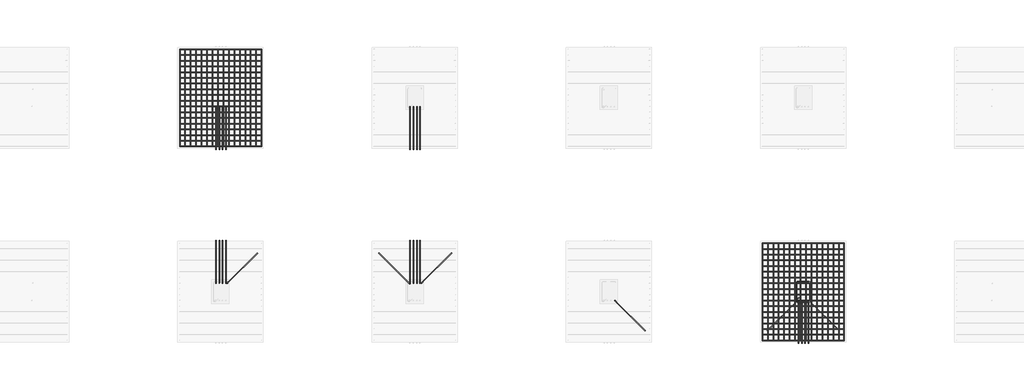
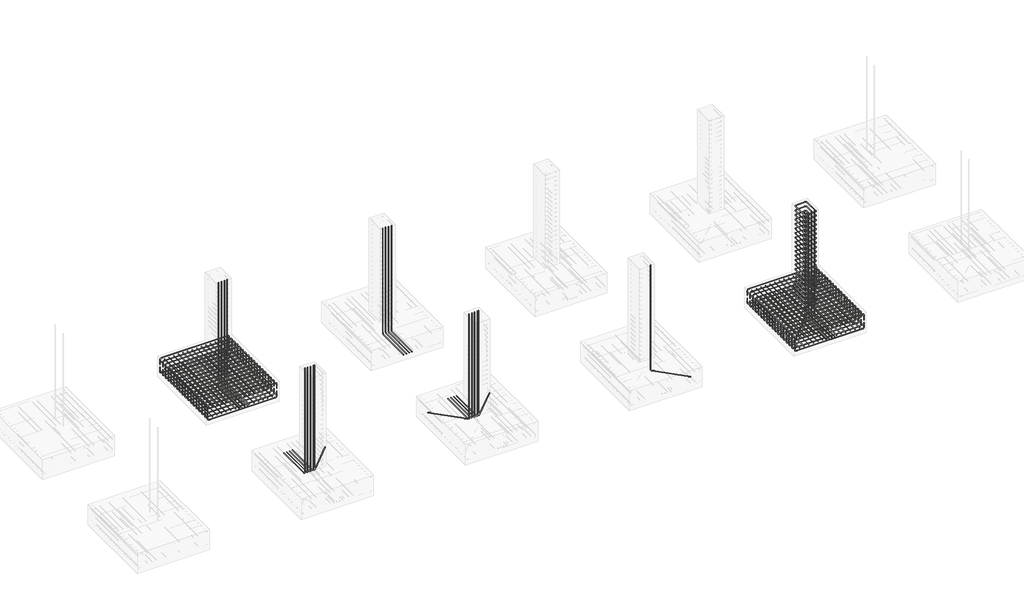
# One storey, part 8 of 33: 20 reinforcing bars.
"""IFC4 building model written with IfcOpenShell, lengths in millimetres."""

from ifc_helpers import new_model, si_unit, point, frame, origin, place, context, project, spatial, polyline, circle_curve, trimmed, segment, composite_curve, source, transform, mapped, element, save
from ifc_brep_helpers import swept_disk

model = new_model("IFC4")

# Units and contexts
model_context = context("Model", 3, world=origin())
ifc_project = project(units=[si_unit("LENGTHUNIT", "METRE", prefix="MILLI")], contexts=[model_context])

# Site, building, storey
site = spatial("IfcSite", under=ifc_project)
building = spatial("IfcBuilding", under=site)
storey = spatial("IfcBuildingStorey", under=building, Elevation=-3000.0)

# Reinforcing bars
placement = place(None, origin())
reinforcing_bar_shape = source(origin(), model_context, "Body", "SolidModel", [
    swept_disk(composite_curve([segment(polyline([(14306.5357258, -7044.0608134, -3240.0), (14306.5357258, -7044.0608134, -3092.7)]), True, "CONTINUOUS"), segment(trimmed(circle_curve(frame((14352.8857258, -7044.0608134, -3092.7), z_axis=(0.0, 1.0, 0.0), x_axis=(-46.350000000000364, 0.0, 0.0)), 46.35), [point((14306.5357258, -7044.0608134, -3092.7))], [point((14352.8857258, -7044.0608134, -3046.35))], True, "CARTESIAN"), True, "CONTINUOUS"), segment(polyline([(14352.8857258, -7044.0608134, -3046.35), (16367.4857258, -7044.0608134, -3046.35)]), True, "CONTINUOUS"), segment(trimmed(circle_curve(frame((16367.4857258, -7044.0608134, -3092.7), z_axis=(0.0, 1.0, 0.0), x_axis=(0.0, 0.0, 46.34999999999991)), 46.35), [point((16367.4857258, -7044.0608134, -3046.35))], [point((16413.8357258, -7044.0608134, -3092.7))], True, "CARTESIAN"), True, "CONTINUOUS"), segment(polyline([(16413.8357258, -7044.0608134, -3092.7), (16413.8357258, -7044.0608134, -3240.0)]), True, "CONTINUOUS")], self_intersect=False), 6.35),
])
element("IfcReinforcingBar", 1, at=placement, inside=storey, context=model_context, shape_type="MappedRepresentation", body=[
    mapped(reinforcing_bar_shape, transform((0.0, 0.0, 0.0), x_axis=(1.0, 0.0, 0.0), y_axis=(0.0, 1.0, 0.0), z_axis=(0.0, 0.0, 1.0))),
    mapped(reinforcing_bar_shape, transform((0.0, -147.4882353, 0.0), x_axis=(1.0, 0.0, 0.0), y_axis=(0.0, 1.0, 0.0), z_axis=(0.0, 0.0, 1.0))),
    mapped(reinforcing_bar_shape, transform((0.0, -294.9764706, 0.0), x_axis=(1.0, 0.0, 0.0), y_axis=(0.0, 1.0, 0.0), z_axis=(0.0, 0.0, 1.0))),
    mapped(reinforcing_bar_shape, transform((0.0, -442.4647059, 0.0), x_axis=(1.0, 0.0, 0.0), y_axis=(0.0, 1.0, 0.0), z_axis=(0.0, 0.0, 1.0))),
    mapped(reinforcing_bar_shape, transform((0.0, -589.9529412, 0.0), x_axis=(1.0, 0.0, 0.0), y_axis=(0.0, 1.0, 0.0), z_axis=(0.0, 0.0, 1.0))),
    mapped(reinforcing_bar_shape, transform((0.0, -737.4411765, 0.0), x_axis=(1.0, 0.0, 0.0), y_axis=(0.0, 1.0, 0.0), z_axis=(0.0, 0.0, 1.0))),
    mapped(reinforcing_bar_shape, transform((0.0, -884.9294118, 0.0), x_axis=(1.0, 0.0, 0.0), y_axis=(0.0, 1.0, 0.0), z_axis=(0.0, 0.0, 1.0))),
    mapped(reinforcing_bar_shape, transform((0.0, -1032.4176471, 0.0), x_axis=(1.0, 0.0, 0.0), y_axis=(0.0, 1.0, 0.0), z_axis=(0.0, 0.0, 1.0))),
    mapped(reinforcing_bar_shape, transform((0.0, -1179.9058824, 0.0), x_axis=(1.0, 0.0, 0.0), y_axis=(0.0, 1.0, 0.0), z_axis=(0.0, 0.0, 1.0))),
    mapped(reinforcing_bar_shape, transform((0.0, -1327.3941176, 0.0), x_axis=(1.0, 0.0, 0.0), y_axis=(0.0, 1.0, 0.0), z_axis=(0.0, 0.0, 1.0))),
    mapped(reinforcing_bar_shape, transform((0.0, -1474.8823529, 0.0), x_axis=(1.0, 0.0, 0.0), y_axis=(0.0, 1.0, 0.0), z_axis=(0.0, 0.0, 1.0))),
    mapped(reinforcing_bar_shape, transform((0.0, -1622.3705882, 0.0), x_axis=(1.0, 0.0, 0.0), y_axis=(0.0, 1.0, 0.0), z_axis=(0.0, 0.0, 1.0))),
    mapped(reinforcing_bar_shape, transform((0.0, -1769.8588235, 0.0), x_axis=(1.0, 0.0, 0.0), y_axis=(0.0, 1.0, 0.0), z_axis=(0.0, 0.0, 1.0))),
    mapped(reinforcing_bar_shape, transform((0.0, -1917.3470588, 0.0), x_axis=(1.0, 0.0, 0.0), y_axis=(0.0, 1.0, 0.0), z_axis=(0.0, 0.0, 1.0))),
    mapped(reinforcing_bar_shape, transform((0.0, -2064.8352941, 0.0), x_axis=(1.0, 0.0, 0.0), y_axis=(0.0, 1.0, 0.0), z_axis=(0.0, 0.0, 1.0))),
    mapped(reinforcing_bar_shape, transform((0.0, -2212.3235294, 0.0), x_axis=(1.0, 0.0, 0.0), y_axis=(0.0, 1.0, 0.0), z_axis=(0.0, 0.0, 1.0))),
    mapped(reinforcing_bar_shape, transform((0.0, -2359.8117647, 0.0), x_axis=(1.0, 0.0, 0.0), y_axis=(0.0, 1.0, 0.0), z_axis=(0.0, 0.0, 1.0))),
    mapped(reinforcing_bar_shape, transform((0.0, -2507.3, 0.0), x_axis=(1.0, 0.0, 0.0), y_axis=(0.0, 1.0, 0.0), z_axis=(0.0, 0.0, 1.0))),
])
reinforcing_bar_2_shape = source(origin(), model_context, "Body", "SolidModel", [
    swept_disk(composite_curve([segment(polyline([(16413.8357258, -7044.0608134, -3330.080452), (16413.8357258, -7044.0608134, -3477.380452)]), True, "CONTINUOUS"), segment(trimmed(circle_curve(frame((16367.4857258, -7044.0608134, -3477.380452), z_axis=(0.0, 1.0, 0.0), x_axis=(46.350000000000364, 0.0, 0.0)), 46.35), [point((16413.8357258, -7044.0608134, -3477.380452))], [point((16367.4857258, -7044.0608134, -3523.730452))], True, "CARTESIAN"), True, "CONTINUOUS"), segment(polyline([(16367.4857258, -7044.0608134, -3523.730452), (14352.8857258, -7044.0608134, -3523.730452)]), True, "CONTINUOUS"), segment(trimmed(circle_curve(frame((14352.8857258, -7044.0608134, -3477.380452), z_axis=(0.0, 1.0, 0.0), x_axis=(0.0, 0.0, -46.34999999999991)), 46.35), [point((14352.8857258, -7044.0608134, -3523.730452))], [point((14306.5357258, -7044.0608134, -3477.380452))], True, "CARTESIAN"), True, "CONTINUOUS"), segment(polyline([(14306.5357258, -7044.0608134, -3477.380452), (14306.5357258, -7044.0608134, -3330.080452)]), True, "CONTINUOUS")], self_intersect=False), 6.35),
])
element("IfcReinforcingBar", 2, at=placement, inside=storey, context=model_context, shape_type="MappedRepresentation", body=[
    mapped(reinforcing_bar_2_shape, transform((0.0, 0.0, 0.0), x_axis=(1.0, 0.0, 0.0), y_axis=(0.0, 1.0, 0.0), z_axis=(0.0, 0.0, 1.0))),
    mapped(reinforcing_bar_2_shape, transform((0.0, -147.4882353, 0.0), x_axis=(1.0, 0.0, 0.0), y_axis=(0.0, 1.0, 0.0), z_axis=(0.0, 0.0, 1.0))),
    mapped(reinforcing_bar_2_shape, transform((0.0, -294.9764706, 0.0), x_axis=(1.0, 0.0, 0.0), y_axis=(0.0, 1.0, 0.0), z_axis=(0.0, 0.0, 1.0))),
    mapped(reinforcing_bar_2_shape, transform((0.0, -442.4647059, 0.0), x_axis=(1.0, 0.0, 0.0), y_axis=(0.0, 1.0, 0.0), z_axis=(0.0, 0.0, 1.0))),
    mapped(reinforcing_bar_2_shape, transform((0.0, -589.9529412, 0.0), x_axis=(1.0, 0.0, 0.0), y_axis=(0.0, 1.0, 0.0), z_axis=(0.0, 0.0, 1.0))),
    mapped(reinforcing_bar_2_shape, transform((0.0, -737.4411765, 0.0), x_axis=(1.0, 0.0, 0.0), y_axis=(0.0, 1.0, 0.0), z_axis=(0.0, 0.0, 1.0))),
    mapped(reinforcing_bar_2_shape, transform((0.0, -884.9294118, 0.0), x_axis=(1.0, 0.0, 0.0), y_axis=(0.0, 1.0, 0.0), z_axis=(0.0, 0.0, 1.0))),
    mapped(reinforcing_bar_2_shape, transform((0.0, -1032.4176471, 0.0), x_axis=(1.0, 0.0, 0.0), y_axis=(0.0, 1.0, 0.0), z_axis=(0.0, 0.0, 1.0))),
    mapped(reinforcing_bar_2_shape, transform((0.0, -1179.9058824, 0.0), x_axis=(1.0, 0.0, 0.0), y_axis=(0.0, 1.0, 0.0), z_axis=(0.0, 0.0, 1.0))),
    mapped(reinforcing_bar_2_shape, transform((0.0, -1327.3941176, 0.0), x_axis=(1.0, 0.0, 0.0), y_axis=(0.0, 1.0, 0.0), z_axis=(0.0, 0.0, 1.0))),
    mapped(reinforcing_bar_2_shape, transform((0.0, -1474.8823529, 0.0), x_axis=(1.0, 0.0, 0.0), y_axis=(0.0, 1.0, 0.0), z_axis=(0.0, 0.0, 1.0))),
    mapped(reinforcing_bar_2_shape, transform((0.0, -1622.3705882, 0.0), x_axis=(1.0, 0.0, 0.0), y_axis=(0.0, 1.0, 0.0), z_axis=(0.0, 0.0, 1.0))),
    mapped(reinforcing_bar_2_shape, transform((0.0, -1769.8588235, 0.0), x_axis=(1.0, 0.0, 0.0), y_axis=(0.0, 1.0, 0.0), z_axis=(0.0, 0.0, 1.0))),
    mapped(reinforcing_bar_2_shape, transform((0.0, -1917.3470588, 0.0), x_axis=(1.0, 0.0, 0.0), y_axis=(0.0, 1.0, 0.0), z_axis=(0.0, 0.0, 1.0))),
    mapped(reinforcing_bar_2_shape, transform((0.0, -2064.8352941, 0.0), x_axis=(1.0, 0.0, 0.0), y_axis=(0.0, 1.0, 0.0), z_axis=(0.0, 0.0, 1.0))),
    mapped(reinforcing_bar_2_shape, transform((0.0, -2212.3235294, 0.0), x_axis=(1.0, 0.0, 0.0), y_axis=(0.0, 1.0, 0.0), z_axis=(0.0, 0.0, 1.0))),
    mapped(reinforcing_bar_2_shape, transform((0.0, -2359.8117647, 0.0), x_axis=(1.0, 0.0, 0.0), y_axis=(0.0, 1.0, 0.0), z_axis=(0.0, 0.0, 1.0))),
    mapped(reinforcing_bar_2_shape, transform((0.0, -2507.3, 0.0), x_axis=(1.0, 0.0, 0.0), y_axis=(0.0, 1.0, 0.0), z_axis=(0.0, 0.0, 1.0))),
])
reinforcing_bar_3_shape = source(origin(), model_context, "Body", "SolidModel", [
    swept_disk(composite_curve([segment(polyline([(16413.8357258, -9557.7108134, -3447.8614173), (16413.8357258, -7037.7108134, -3447.8614173)]), True, "CONTINUOUS")], self_intersect=False), 6.35),
])
element("IfcReinforcingBar", 3, at=placement, inside=storey, context=model_context, shape_type="MappedRepresentation", body=[
    mapped(reinforcing_bar_3_shape, transform((0.0, 0.0, 0.0), x_axis=(1.0, 0.0, 0.0), y_axis=(0.0, 1.0, 0.0), z_axis=(0.0, 0.0, 1.0))),
    mapped(reinforcing_bar_3_shape, transform((-140.4866667, 0.0, 0.0), x_axis=(1.0, 0.0, 0.0), y_axis=(0.0, 1.0, 0.0), z_axis=(0.0, 0.0, 1.0))),
    mapped(reinforcing_bar_3_shape, transform((-280.9733333, 0.0, 0.0), x_axis=(1.0, 0.0, 0.0), y_axis=(0.0, 1.0, 0.0), z_axis=(0.0, 0.0, 1.0))),
    mapped(reinforcing_bar_3_shape, transform((-421.46, 0.0, 0.0), x_axis=(1.0, 0.0, 0.0), y_axis=(0.0, 1.0, 0.0), z_axis=(0.0, 0.0, 1.0))),
    mapped(reinforcing_bar_3_shape, transform((-561.9466667, 0.0, 0.0), x_axis=(1.0, 0.0, 0.0), y_axis=(0.0, 1.0, 0.0), z_axis=(0.0, 0.0, 1.0))),
    mapped(reinforcing_bar_3_shape, transform((-702.4333333, 0.0, 0.0), x_axis=(1.0, 0.0, 0.0), y_axis=(0.0, 1.0, 0.0), z_axis=(0.0, 0.0, 1.0))),
    mapped(reinforcing_bar_3_shape, transform((-842.92, 0.0, 0.0), x_axis=(1.0, 0.0, 0.0), y_axis=(0.0, 1.0, 0.0), z_axis=(0.0, 0.0, 1.0))),
    mapped(reinforcing_bar_3_shape, transform((-983.4066667, 0.0, 0.0), x_axis=(1.0, 0.0, 0.0), y_axis=(0.0, 1.0, 0.0), z_axis=(0.0, 0.0, 1.0))),
    mapped(reinforcing_bar_3_shape, transform((-1123.8933333, 0.0, 0.0), x_axis=(1.0, 0.0, 0.0), y_axis=(0.0, 1.0, 0.0), z_axis=(0.0, 0.0, 1.0))),
    mapped(reinforcing_bar_3_shape, transform((-1264.38, 0.0, 0.0), x_axis=(1.0, 0.0, 0.0), y_axis=(0.0, 1.0, 0.0), z_axis=(0.0, 0.0, 1.0))),
    mapped(reinforcing_bar_3_shape, transform((-1404.8666667, 0.0, 0.0), x_axis=(1.0, 0.0, 0.0), y_axis=(0.0, 1.0, 0.0), z_axis=(0.0, 0.0, 1.0))),
    mapped(reinforcing_bar_3_shape, transform((-1545.3533333, 0.0, 0.0), x_axis=(1.0, 0.0, 0.0), y_axis=(0.0, 1.0, 0.0), z_axis=(0.0, 0.0, 1.0))),
    mapped(reinforcing_bar_3_shape, transform((-1685.84, 0.0, 0.0), x_axis=(1.0, 0.0, 0.0), y_axis=(0.0, 1.0, 0.0), z_axis=(0.0, 0.0, 1.0))),
    mapped(reinforcing_bar_3_shape, transform((-1826.3266667, 0.0, 0.0), x_axis=(1.0, 0.0, 0.0), y_axis=(0.0, 1.0, 0.0), z_axis=(0.0, 0.0, 1.0))),
    mapped(reinforcing_bar_3_shape, transform((-1966.8133333, 0.0, 0.0), x_axis=(1.0, 0.0, 0.0), y_axis=(0.0, 1.0, 0.0), z_axis=(0.0, 0.0, 1.0))),
    mapped(reinforcing_bar_3_shape, transform((-2107.3, 0.0, 0.0), x_axis=(1.0, 0.0, 0.0), y_axis=(0.0, 1.0, 0.0), z_axis=(0.0, 0.0, 1.0))),
])
reinforcing_bar_4_shape = source(origin(), model_context, "Body", "SolidModel", [
    swept_disk(composite_curve([segment(polyline([(14306.5357258, -9557.7108134, -3122.7084113), (14306.5357258, -7037.7108134, -3122.7084113)]), True, "CONTINUOUS")], self_intersect=False), 6.35),
])
element("IfcReinforcingBar", 4, at=placement, inside=storey, context=model_context, shape_type="MappedRepresentation", body=[
    mapped(reinforcing_bar_4_shape, transform((0.0, 0.0, 0.0), x_axis=(1.0, 0.0, 0.0), y_axis=(0.0, 1.0, 0.0), z_axis=(0.0, 0.0, 1.0))),
    mapped(reinforcing_bar_4_shape, transform((140.4866667, 0.0, 0.0), x_axis=(1.0, 0.0, 0.0), y_axis=(0.0, 1.0, 0.0), z_axis=(0.0, 0.0, 1.0))),
    mapped(reinforcing_bar_4_shape, transform((280.9733333, 0.0, 0.0), x_axis=(1.0, 0.0, 0.0), y_axis=(0.0, 1.0, 0.0), z_axis=(0.0, 0.0, 1.0))),
    mapped(reinforcing_bar_4_shape, transform((421.46, 0.0, 0.0), x_axis=(1.0, 0.0, 0.0), y_axis=(0.0, 1.0, 0.0), z_axis=(0.0, 0.0, 1.0))),
    mapped(reinforcing_bar_4_shape, transform((561.9466667, 0.0, 0.0), x_axis=(1.0, 0.0, 0.0), y_axis=(0.0, 1.0, 0.0), z_axis=(0.0, 0.0, 1.0))),
    mapped(reinforcing_bar_4_shape, transform((702.4333333, 0.0, 0.0), x_axis=(1.0, 0.0, 0.0), y_axis=(0.0, 1.0, 0.0), z_axis=(0.0, 0.0, 1.0))),
    mapped(reinforcing_bar_4_shape, transform((842.92, 0.0, 0.0), x_axis=(1.0, 0.0, 0.0), y_axis=(0.0, 1.0, 0.0), z_axis=(0.0, 0.0, 1.0))),
    mapped(reinforcing_bar_4_shape, transform((983.4066667, 0.0, 0.0), x_axis=(1.0, 0.0, 0.0), y_axis=(0.0, 1.0, 0.0), z_axis=(0.0, 0.0, 1.0))),
    mapped(reinforcing_bar_4_shape, transform((1123.8933333, 0.0, 0.0), x_axis=(1.0, 0.0, 0.0), y_axis=(0.0, 1.0, 0.0), z_axis=(0.0, 0.0, 1.0))),
    mapped(reinforcing_bar_4_shape, transform((1264.38, 0.0, 0.0), x_axis=(1.0, 0.0, 0.0), y_axis=(0.0, 1.0, 0.0), z_axis=(0.0, 0.0, 1.0))),
    mapped(reinforcing_bar_4_shape, transform((1404.8666667, 0.0, 0.0), x_axis=(1.0, 0.0, 0.0), y_axis=(0.0, 1.0, 0.0), z_axis=(0.0, 0.0, 1.0))),
    mapped(reinforcing_bar_4_shape, transform((1545.3533333, 0.0, 0.0), x_axis=(1.0, 0.0, 0.0), y_axis=(0.0, 1.0, 0.0), z_axis=(0.0, 0.0, 1.0))),
    mapped(reinforcing_bar_4_shape, transform((1685.84, 0.0, 0.0), x_axis=(1.0, 0.0, 0.0), y_axis=(0.0, 1.0, 0.0), z_axis=(0.0, 0.0, 1.0))),
    mapped(reinforcing_bar_4_shape, transform((1826.3266667, 0.0, 0.0), x_axis=(1.0, 0.0, 0.0), y_axis=(0.0, 1.0, 0.0), z_axis=(0.0, 0.0, 1.0))),
    mapped(reinforcing_bar_4_shape, transform((1966.8133333, 0.0, 0.0), x_axis=(1.0, 0.0, 0.0), y_axis=(0.0, 1.0, 0.0), z_axis=(0.0, 0.0, 1.0))),
    mapped(reinforcing_bar_4_shape, transform((2107.3, 0.0, 0.0), x_axis=(1.0, 0.0, 0.0), y_axis=(0.0, 1.0, 0.0), z_axis=(0.0, 0.0, 1.0))),
])
reinforcing_bar_5_shape = source(origin(), model_context, "Body", "SolidModel", [
    swept_disk(composite_curve([segment(polyline([(-693.4642742, -2044.0608134, -3240.0), (-693.4642742, -2044.0608134, -3092.7)]), True, "CONTINUOUS"), segment(trimmed(circle_curve(frame((-647.1142742, -2044.0608134, -3092.7), z_axis=(0.0, 1.0, 0.0), x_axis=(-46.35000000000002, 0.0, 0.0)), 46.35), [point((-693.4642742, -2044.0608134, -3092.7))], [point((-647.1142742, -2044.0608134, -3046.35))], True, "CARTESIAN"), True, "CONTINUOUS"), segment(polyline([(-647.1142742, -2044.0608134, -3046.35), (1367.4857258, -2044.0608134, -3046.35)]), True, "CONTINUOUS"), segment(trimmed(circle_curve(frame((1367.4857258, -2044.0608134, -3092.7), z_axis=(0.0, 1.0, 0.0), x_axis=(0.0, 0.0, 46.34999999999991)), 46.35), [point((1367.4857258, -2044.0608134, -3046.35))], [point((1413.8357258, -2044.0608134, -3092.7))], True, "CARTESIAN"), True, "CONTINUOUS"), segment(polyline([(1413.8357258, -2044.0608134, -3092.7), (1413.8357258, -2044.0608134, -3240.0)]), True, "CONTINUOUS")], self_intersect=False), 6.35),
])
element("IfcReinforcingBar", 5, at=placement, inside=storey, context=model_context, shape_type="MappedRepresentation", body=[
    mapped(reinforcing_bar_5_shape, transform((0.0, 0.0, 0.0), x_axis=(1.0, 0.0, 0.0), y_axis=(0.0, 1.0, 0.0), z_axis=(0.0, 0.0, 1.0))),
    mapped(reinforcing_bar_5_shape, transform((0.0, -147.4882353, 0.0), x_axis=(1.0, 0.0, 0.0), y_axis=(0.0, 1.0, 0.0), z_axis=(0.0, 0.0, 1.0))),
    mapped(reinforcing_bar_5_shape, transform((0.0, -294.9764706, 0.0), x_axis=(1.0, 0.0, 0.0), y_axis=(0.0, 1.0, 0.0), z_axis=(0.0, 0.0, 1.0))),
    mapped(reinforcing_bar_5_shape, transform((0.0, -442.4647059, 0.0), x_axis=(1.0, 0.0, 0.0), y_axis=(0.0, 1.0, 0.0), z_axis=(0.0, 0.0, 1.0))),
    mapped(reinforcing_bar_5_shape, transform((0.0, -589.9529412, 0.0), x_axis=(1.0, 0.0, 0.0), y_axis=(0.0, 1.0, 0.0), z_axis=(0.0, 0.0, 1.0))),
    mapped(reinforcing_bar_5_shape, transform((0.0, -737.4411765, 0.0), x_axis=(1.0, 0.0, 0.0), y_axis=(0.0, 1.0, 0.0), z_axis=(0.0, 0.0, 1.0))),
    mapped(reinforcing_bar_5_shape, transform((0.0, -884.9294118, 0.0), x_axis=(1.0, 0.0, 0.0), y_axis=(0.0, 1.0, 0.0), z_axis=(0.0, 0.0, 1.0))),
    mapped(reinforcing_bar_5_shape, transform((0.0, -1032.4176471, 0.0), x_axis=(1.0, 0.0, 0.0), y_axis=(0.0, 1.0, 0.0), z_axis=(0.0, 0.0, 1.0))),
    mapped(reinforcing_bar_5_shape, transform((0.0, -1179.9058824, 0.0), x_axis=(1.0, 0.0, 0.0), y_axis=(0.0, 1.0, 0.0), z_axis=(0.0, 0.0, 1.0))),
    mapped(reinforcing_bar_5_shape, transform((0.0, -1327.3941176, 0.0), x_axis=(1.0, 0.0, 0.0), y_axis=(0.0, 1.0, 0.0), z_axis=(0.0, 0.0, 1.0))),
    mapped(reinforcing_bar_5_shape, transform((0.0, -1474.8823529, 0.0), x_axis=(1.0, 0.0, 0.0), y_axis=(0.0, 1.0, 0.0), z_axis=(0.0, 0.0, 1.0))),
    mapped(reinforcing_bar_5_shape, transform((0.0, -1622.3705882, 0.0), x_axis=(1.0, 0.0, 0.0), y_axis=(0.0, 1.0, 0.0), z_axis=(0.0, 0.0, 1.0))),
    mapped(reinforcing_bar_5_shape, transform((0.0, -1769.8588235, 0.0), x_axis=(1.0, 0.0, 0.0), y_axis=(0.0, 1.0, 0.0), z_axis=(0.0, 0.0, 1.0))),
    mapped(reinforcing_bar_5_shape, transform((0.0, -1917.3470588, 0.0), x_axis=(1.0, 0.0, 0.0), y_axis=(0.0, 1.0, 0.0), z_axis=(0.0, 0.0, 1.0))),
    mapped(reinforcing_bar_5_shape, transform((0.0, -2064.8352941, 0.0), x_axis=(1.0, 0.0, 0.0), y_axis=(0.0, 1.0, 0.0), z_axis=(0.0, 0.0, 1.0))),
    mapped(reinforcing_bar_5_shape, transform((0.0, -2212.3235294, 0.0), x_axis=(1.0, 0.0, 0.0), y_axis=(0.0, 1.0, 0.0), z_axis=(0.0, 0.0, 1.0))),
    mapped(reinforcing_bar_5_shape, transform((0.0, -2359.8117647, 0.0), x_axis=(1.0, 0.0, 0.0), y_axis=(0.0, 1.0, 0.0), z_axis=(0.0, 0.0, 1.0))),
    mapped(reinforcing_bar_5_shape, transform((0.0, -2507.3, 0.0), x_axis=(1.0, 0.0, 0.0), y_axis=(0.0, 1.0, 0.0), z_axis=(0.0, 0.0, 1.0))),
])
reinforcing_bar_6_shape = source(origin(), model_context, "Body", "SolidModel", [
    swept_disk(composite_curve([segment(polyline([(1413.8357258, -2044.0608134, -3330.080452), (1413.8357258, -2044.0608134, -3477.380452)]), True, "CONTINUOUS"), segment(trimmed(circle_curve(frame((1367.4857258, -2044.0608134, -3477.380452), z_axis=(0.0, 1.0, 0.0), x_axis=(46.350000000000136, 0.0, 0.0)), 46.35), [point((1413.8357258, -2044.0608134, -3477.380452))], [point((1367.4857258, -2044.0608134, -3523.730452))], True, "CARTESIAN"), True, "CONTINUOUS"), segment(polyline([(1367.4857258, -2044.0608134, -3523.730452), (-647.1142742, -2044.0608134, -3523.730452)]), True, "CONTINUOUS"), segment(trimmed(circle_curve(frame((-647.1142742, -2044.0608134, -3477.380452), z_axis=(0.0, 1.0, 0.0), x_axis=(0.0, 0.0, -46.34999999999991)), 46.35), [point((-647.1142742, -2044.0608134, -3523.730452))], [point((-693.4642742, -2044.0608134, -3477.380452))], True, "CARTESIAN"), True, "CONTINUOUS"), segment(polyline([(-693.4642742, -2044.0608134, -3477.380452), (-693.4642742, -2044.0608134, -3330.080452)]), True, "CONTINUOUS")], self_intersect=False), 6.35),
])
element("IfcReinforcingBar", 6, at=placement, inside=storey, context=model_context, shape_type="MappedRepresentation", body=[
    mapped(reinforcing_bar_6_shape, transform((0.0, 0.0, 0.0), x_axis=(1.0, 0.0, 0.0), y_axis=(0.0, 1.0, 0.0), z_axis=(0.0, 0.0, 1.0))),
    mapped(reinforcing_bar_6_shape, transform((0.0, -147.4882353, 0.0), x_axis=(1.0, 0.0, 0.0), y_axis=(0.0, 1.0, 0.0), z_axis=(0.0, 0.0, 1.0))),
    mapped(reinforcing_bar_6_shape, transform((0.0, -294.9764706, 0.0), x_axis=(1.0, 0.0, 0.0), y_axis=(0.0, 1.0, 0.0), z_axis=(0.0, 0.0, 1.0))),
    mapped(reinforcing_bar_6_shape, transform((0.0, -442.4647059, 0.0), x_axis=(1.0, 0.0, 0.0), y_axis=(0.0, 1.0, 0.0), z_axis=(0.0, 0.0, 1.0))),
    mapped(reinforcing_bar_6_shape, transform((0.0, -589.9529412, 0.0), x_axis=(1.0, 0.0, 0.0), y_axis=(0.0, 1.0, 0.0), z_axis=(0.0, 0.0, 1.0))),
    mapped(reinforcing_bar_6_shape, transform((0.0, -737.4411765, 0.0), x_axis=(1.0, 0.0, 0.0), y_axis=(0.0, 1.0, 0.0), z_axis=(0.0, 0.0, 1.0))),
    mapped(reinforcing_bar_6_shape, transform((0.0, -884.9294118, 0.0), x_axis=(1.0, 0.0, 0.0), y_axis=(0.0, 1.0, 0.0), z_axis=(0.0, 0.0, 1.0))),
    mapped(reinforcing_bar_6_shape, transform((0.0, -1032.4176471, 0.0), x_axis=(1.0, 0.0, 0.0), y_axis=(0.0, 1.0, 0.0), z_axis=(0.0, 0.0, 1.0))),
    mapped(reinforcing_bar_6_shape, transform((0.0, -1179.9058824, 0.0), x_axis=(1.0, 0.0, 0.0), y_axis=(0.0, 1.0, 0.0), z_axis=(0.0, 0.0, 1.0))),
    mapped(reinforcing_bar_6_shape, transform((0.0, -1327.3941176, 0.0), x_axis=(1.0, 0.0, 0.0), y_axis=(0.0, 1.0, 0.0), z_axis=(0.0, 0.0, 1.0))),
    mapped(reinforcing_bar_6_shape, transform((0.0, -1474.8823529, 0.0), x_axis=(1.0, 0.0, 0.0), y_axis=(0.0, 1.0, 0.0), z_axis=(0.0, 0.0, 1.0))),
    mapped(reinforcing_bar_6_shape, transform((0.0, -1622.3705882, 0.0), x_axis=(1.0, 0.0, 0.0), y_axis=(0.0, 1.0, 0.0), z_axis=(0.0, 0.0, 1.0))),
    mapped(reinforcing_bar_6_shape, transform((0.0, -1769.8588235, 0.0), x_axis=(1.0, 0.0, 0.0), y_axis=(0.0, 1.0, 0.0), z_axis=(0.0, 0.0, 1.0))),
    mapped(reinforcing_bar_6_shape, transform((0.0, -1917.3470588, 0.0), x_axis=(1.0, 0.0, 0.0), y_axis=(0.0, 1.0, 0.0), z_axis=(0.0, 0.0, 1.0))),
    mapped(reinforcing_bar_6_shape, transform((0.0, -2064.8352941, 0.0), x_axis=(1.0, 0.0, 0.0), y_axis=(0.0, 1.0, 0.0), z_axis=(0.0, 0.0, 1.0))),
    mapped(reinforcing_bar_6_shape, transform((0.0, -2212.3235294, 0.0), x_axis=(1.0, 0.0, 0.0), y_axis=(0.0, 1.0, 0.0), z_axis=(0.0, 0.0, 1.0))),
    mapped(reinforcing_bar_6_shape, transform((0.0, -2359.8117647, 0.0), x_axis=(1.0, 0.0, 0.0), y_axis=(0.0, 1.0, 0.0), z_axis=(0.0, 0.0, 1.0))),
    mapped(reinforcing_bar_6_shape, transform((0.0, -2507.3, 0.0), x_axis=(1.0, 0.0, 0.0), y_axis=(0.0, 1.0, 0.0), z_axis=(0.0, 0.0, 1.0))),
])
reinforcing_bar_7_shape = source(origin(), model_context, "Body", "SolidModel", [
    swept_disk(composite_curve([segment(polyline([(1413.8357258, -4557.7108134, -3447.8614173), (1413.8357258, -2037.7108134, -3447.8614173)]), True, "CONTINUOUS")], self_intersect=False), 6.35),
])
element("IfcReinforcingBar", 7, at=placement, inside=storey, context=model_context, shape_type="MappedRepresentation", body=[
    mapped(reinforcing_bar_7_shape, transform((0.0, 0.0, 0.0), x_axis=(1.0, 0.0, 0.0), y_axis=(0.0, 1.0, 0.0), z_axis=(0.0, 0.0, 1.0))),
    mapped(reinforcing_bar_7_shape, transform((-140.4866667, 0.0, 0.0), x_axis=(1.0, 0.0, 0.0), y_axis=(0.0, 1.0, 0.0), z_axis=(0.0, 0.0, 1.0))),
    mapped(reinforcing_bar_7_shape, transform((-280.9733333, 0.0, 0.0), x_axis=(1.0, 0.0, 0.0), y_axis=(0.0, 1.0, 0.0), z_axis=(0.0, 0.0, 1.0))),
    mapped(reinforcing_bar_7_shape, transform((-421.46, 0.0, 0.0), x_axis=(1.0, 0.0, 0.0), y_axis=(0.0, 1.0, 0.0), z_axis=(0.0, 0.0, 1.0))),
    mapped(reinforcing_bar_7_shape, transform((-561.9466667, 0.0, 0.0), x_axis=(1.0, 0.0, 0.0), y_axis=(0.0, 1.0, 0.0), z_axis=(0.0, 0.0, 1.0))),
    mapped(reinforcing_bar_7_shape, transform((-702.4333333, 0.0, 0.0), x_axis=(1.0, 0.0, 0.0), y_axis=(0.0, 1.0, 0.0), z_axis=(0.0, 0.0, 1.0))),
    mapped(reinforcing_bar_7_shape, transform((-842.92, 0.0, 0.0), x_axis=(1.0, 0.0, 0.0), y_axis=(0.0, 1.0, 0.0), z_axis=(0.0, 0.0, 1.0))),
    mapped(reinforcing_bar_7_shape, transform((-983.4066667, 0.0, 0.0), x_axis=(1.0, 0.0, 0.0), y_axis=(0.0, 1.0, 0.0), z_axis=(0.0, 0.0, 1.0))),
    mapped(reinforcing_bar_7_shape, transform((-1123.8933333, 0.0, 0.0), x_axis=(1.0, 0.0, 0.0), y_axis=(0.0, 1.0, 0.0), z_axis=(0.0, 0.0, 1.0))),
    mapped(reinforcing_bar_7_shape, transform((-1264.38, 0.0, 0.0), x_axis=(1.0, 0.0, 0.0), y_axis=(0.0, 1.0, 0.0), z_axis=(0.0, 0.0, 1.0))),
    mapped(reinforcing_bar_7_shape, transform((-1404.8666667, 0.0, 0.0), x_axis=(1.0, 0.0, 0.0), y_axis=(0.0, 1.0, 0.0), z_axis=(0.0, 0.0, 1.0))),
    mapped(reinforcing_bar_7_shape, transform((-1545.3533333, 0.0, 0.0), x_axis=(1.0, 0.0, 0.0), y_axis=(0.0, 1.0, 0.0), z_axis=(0.0, 0.0, 1.0))),
    mapped(reinforcing_bar_7_shape, transform((-1685.84, 0.0, 0.0), x_axis=(1.0, 0.0, 0.0), y_axis=(0.0, 1.0, 0.0), z_axis=(0.0, 0.0, 1.0))),
    mapped(reinforcing_bar_7_shape, transform((-1826.3266667, 0.0, 0.0), x_axis=(1.0, 0.0, 0.0), y_axis=(0.0, 1.0, 0.0), z_axis=(0.0, 0.0, 1.0))),
    mapped(reinforcing_bar_7_shape, transform((-1966.8133333, 0.0, 0.0), x_axis=(1.0, 0.0, 0.0), y_axis=(0.0, 1.0, 0.0), z_axis=(0.0, 0.0, 1.0))),
    mapped(reinforcing_bar_7_shape, transform((-2107.3, 0.0, 0.0), x_axis=(1.0, 0.0, 0.0), y_axis=(0.0, 1.0, 0.0), z_axis=(0.0, 0.0, 1.0))),
])
reinforcing_bar_8_shape = source(origin(), model_context, "Body", "SolidModel", [
    swept_disk(composite_curve([segment(polyline([(-693.4642742, -4557.7108134, -3122.7084113), (-693.4642742, -2037.7108134, -3122.7084113)]), True, "CONTINUOUS")], self_intersect=False), 6.35),
])
element("IfcReinforcingBar", 8, at=placement, inside=storey, context=model_context, shape_type="MappedRepresentation", body=[
    mapped(reinforcing_bar_8_shape, transform((0.0, 0.0, 0.0), x_axis=(1.0, 0.0, 0.0), y_axis=(0.0, 1.0, 0.0), z_axis=(0.0, 0.0, 1.0))),
    mapped(reinforcing_bar_8_shape, transform((140.4866667, 0.0, 0.0), x_axis=(1.0, 0.0, 0.0), y_axis=(0.0, 1.0, 0.0), z_axis=(0.0, 0.0, 1.0))),
    mapped(reinforcing_bar_8_shape, transform((280.9733333, 0.0, 0.0), x_axis=(1.0, 0.0, 0.0), y_axis=(0.0, 1.0, 0.0), z_axis=(0.0, 0.0, 1.0))),
    mapped(reinforcing_bar_8_shape, transform((421.46, 0.0, 0.0), x_axis=(1.0, 0.0, 0.0), y_axis=(0.0, 1.0, 0.0), z_axis=(0.0, 0.0, 1.0))),
    mapped(reinforcing_bar_8_shape, transform((561.9466667, 0.0, 0.0), x_axis=(1.0, 0.0, 0.0), y_axis=(0.0, 1.0, 0.0), z_axis=(0.0, 0.0, 1.0))),
    mapped(reinforcing_bar_8_shape, transform((702.4333333, 0.0, 0.0), x_axis=(1.0, 0.0, 0.0), y_axis=(0.0, 1.0, 0.0), z_axis=(0.0, 0.0, 1.0))),
    mapped(reinforcing_bar_8_shape, transform((842.92, 0.0, 0.0), x_axis=(1.0, 0.0, 0.0), y_axis=(0.0, 1.0, 0.0), z_axis=(0.0, 0.0, 1.0))),
    mapped(reinforcing_bar_8_shape, transform((983.4066667, 0.0, 0.0), x_axis=(1.0, 0.0, 0.0), y_axis=(0.0, 1.0, 0.0), z_axis=(0.0, 0.0, 1.0))),
    mapped(reinforcing_bar_8_shape, transform((1123.8933333, 0.0, 0.0), x_axis=(1.0, 0.0, 0.0), y_axis=(0.0, 1.0, 0.0), z_axis=(0.0, 0.0, 1.0))),
    mapped(reinforcing_bar_8_shape, transform((1264.38, 0.0, 0.0), x_axis=(1.0, 0.0, 0.0), y_axis=(0.0, 1.0, 0.0), z_axis=(0.0, 0.0, 1.0))),
    mapped(reinforcing_bar_8_shape, transform((1404.8666667, 0.0, 0.0), x_axis=(1.0, 0.0, 0.0), y_axis=(0.0, 1.0, 0.0), z_axis=(0.0, 0.0, 1.0))),
    mapped(reinforcing_bar_8_shape, transform((1545.3533333, 0.0, 0.0), x_axis=(1.0, 0.0, 0.0), y_axis=(0.0, 1.0, 0.0), z_axis=(0.0, 0.0, 1.0))),
    mapped(reinforcing_bar_8_shape, transform((1685.84, 0.0, 0.0), x_axis=(1.0, 0.0, 0.0), y_axis=(0.0, 1.0, 0.0), z_axis=(0.0, 0.0, 1.0))),
    mapped(reinforcing_bar_8_shape, transform((1826.3266667, 0.0, 0.0), x_axis=(1.0, 0.0, 0.0), y_axis=(0.0, 1.0, 0.0), z_axis=(0.0, 0.0, 1.0))),
    mapped(reinforcing_bar_8_shape, transform((1966.8133333, 0.0, 0.0), x_axis=(1.0, 0.0, 0.0), y_axis=(0.0, 1.0, 0.0), z_axis=(0.0, 0.0, 1.0))),
    mapped(reinforcing_bar_8_shape, transform((2107.3, 0.0, 0.0), x_axis=(1.0, 0.0, 0.0), y_axis=(0.0, 1.0, 0.0), z_axis=(0.0, 0.0, 1.0))),
])
reinforcing_bar_9_shape = source(origin(), model_context, "Body", "SolidModel", [
    swept_disk(composite_curve([segment(polyline([(236.1158322, -3523.4938134, -40.0), (236.1158322, -3523.4938134, -3393.65)]), True, "CONTINUOUS"), segment(trimmed(circle_curve(frame((236.1158322, -3569.8438134, -3393.65), z_axis=(-1.0, 0.0, 0.0), x_axis=(0.0, 46.34999999999991, 0.0)), 46.35), [point((236.1158322, -3523.4938134, -3393.65))], [point((236.1158322, -3569.8438134, -3440.0))], True, "CARTESIAN"), True, "CONTINUOUS"), segment(polyline([(236.1158322, -3569.8438134, -3440.0), (236.1158322, -4623.4938134, -3440.0)]), True, "CONTINUOUS")], self_intersect=False), 6.35),
])
element("IfcReinforcingBar", 9, at=placement, inside=storey, context=model_context, shape_type="MappedRepresentation", body=[
    mapped(reinforcing_bar_9_shape, transform((0.0, 0.0, 0.0), x_axis=(1.0, 0.0, 0.0), y_axis=(0.0, 1.0, 0.0), z_axis=(0.0, 0.0, 1.0))),
    mapped(reinforcing_bar_9_shape, transform((86.8979716, 0.0, 0.0), x_axis=(1.0, 0.0, 0.0), y_axis=(0.0, 1.0, 0.0), z_axis=(0.0, 0.0, 1.0))),
    mapped(reinforcing_bar_9_shape, transform((173.7959432, 0.0, 0.0), x_axis=(1.0, 0.0, 0.0), y_axis=(0.0, 1.0, 0.0), z_axis=(0.0, 0.0, 1.0))),
    mapped(reinforcing_bar_9_shape, transform((260.6939148, 0.0, 0.0), x_axis=(1.0, 0.0, 0.0), y_axis=(0.0, 1.0, 0.0), z_axis=(0.0, 0.0, 1.0))),
])
element("IfcReinforcingBar", 10, at=placement, inside=storey, context=model_context, shape_type="SolidModel", body=[
    swept_disk(composite_curve([segment(polyline([(525.7684217, -8073.7876853, -30.2564663), (525.7684217, -8073.7876853, -3383.9064663)]), True, "CONTINUOUS"), segment(trimmed(circle_curve(frame((558.542821, -8041.013286, -3383.9064663), z_axis=(0.7071067811865493, -0.7071067811865459, 0.0), x_axis=(-32.77439930000003, -32.77439929999946, 0.0)), 46.35), [point((525.7684217, -8073.7876853, -3383.9064663))], [point((558.542821, -8041.013286, -3430.2564663))], True, "CARTESIAN"), True, "CONTINUOUS"), segment(polyline([(558.542821, -8041.013286, -3430.2564663), (1303.585881, -7295.970226, -3430.2564663)]), True, "CONTINUOUS")], self_intersect=False), 6.35),
])
reinforcing_bar_10_shape = source(origin(), model_context, "Body", "SolidModel", [
    swept_disk(composite_curve([segment(polyline([(236.1158322, -8071.9278134, -40.0), (236.1158322, -8071.9278134, -3393.65)]), True, "CONTINUOUS"), segment(trimmed(circle_curve(frame((236.1158322, -8025.5778134, -3393.65), z_axis=(1.0, 0.0, 0.0), x_axis=(0.0, -46.349999999999454, 0.0)), 46.35), [point((236.1158322, -8071.9278134, -3393.65))], [point((236.1158322, -8025.5778134, -3440.0))], True, "CARTESIAN"), True, "CONTINUOUS"), segment(polyline([(236.1158322, -8025.5778134, -3440.0), (236.1158322, -6971.9278134, -3440.0)]), True, "CONTINUOUS")], self_intersect=False), 6.35),
])
element("IfcReinforcingBar", 11, at=placement, inside=storey, context=model_context, shape_type="MappedRepresentation", body=[
    mapped(reinforcing_bar_10_shape, transform((0.0, 0.0, 0.0), x_axis=(1.0, 0.0, 0.0), y_axis=(0.0, 1.0, 0.0), z_axis=(0.0, 0.0, 1.0))),
    mapped(reinforcing_bar_10_shape, transform((86.8979716, 0.0, 0.0), x_axis=(1.0, 0.0, 0.0), y_axis=(0.0, 1.0, 0.0), z_axis=(0.0, 0.0, 1.0))),
    mapped(reinforcing_bar_10_shape, transform((173.7959432, 0.0, 0.0), x_axis=(1.0, 0.0, 0.0), y_axis=(0.0, 1.0, 0.0), z_axis=(0.0, 0.0, 1.0))),
    mapped(reinforcing_bar_10_shape, transform((260.6939148, 0.0, 0.0), x_axis=(1.0, 0.0, 0.0), y_axis=(0.0, 1.0, 0.0), z_axis=(0.0, 0.0, 1.0))),
])
element("IfcReinforcingBar", 12, at=placement, inside=storey, context=model_context, shape_type="SolidModel", body=[
    swept_disk(composite_curve([segment(polyline([(5231.1024274, -8091.6857913, -40.0), (5231.1024274, -8091.6857913, -3361.434517)]), True, "CONTINUOUS"), segment(trimmed(circle_curve(frame((5198.3280281, -8058.911392, -3361.434517), z_axis=(0.7071067811865539, 0.7071067811865411, 0.0), x_axis=(32.77439930000037, -32.77439930000037, 0.0)), 46.35), [point((5231.1024274, -8091.6857913, -3361.434517))], [point((5198.3280281, -8058.911392, -3407.784517))], True, "CARTESIAN"), True, "CONTINUOUS"), segment(polyline([(5198.3280281, -8058.911392, -3407.784517), (4435.3868621, -7295.970226, -3407.784517)]), True, "CONTINUOUS")], self_intersect=False), 6.35),
])
element("IfcReinforcingBar", 13, at=placement, inside=storey, context=model_context, shape_type="SolidModel", body=[
    swept_disk(composite_curve([segment(polyline([(5525.7684217, -8073.7876853, -30.2564663), (5525.7684217, -8073.7876853, -3383.9064663)]), True, "CONTINUOUS"), segment(trimmed(circle_curve(frame((5558.542821, -8041.013286, -3383.9064663), z_axis=(0.7071067811865493, -0.7071067811865459, 0.0), x_axis=(-32.77439930000037, -32.77439929999946, 0.0)), 46.35), [point((5525.7684217, -8073.7876853, -3383.9064663))], [point((5558.542821, -8041.013286, -3430.2564663))], True, "CARTESIAN"), True, "CONTINUOUS"), segment(polyline([(5558.542821, -8041.013286, -3430.2564663), (6303.585881, -7295.970226, -3430.2564663)]), True, "CONTINUOUS")], self_intersect=False), 6.35),
])
reinforcing_bar_11_shape = source(origin(), model_context, "Body", "SolidModel", [
    swept_disk(composite_curve([segment(polyline([(5236.1158322, -8071.9278134, -40.0), (5236.1158322, -8071.9278134, -3393.65)]), True, "CONTINUOUS"), segment(trimmed(circle_curve(frame((5236.1158322, -8025.5778134, -3393.65), z_axis=(1.0, 0.0, 0.0), x_axis=(0.0, -46.349999999999454, 0.0)), 46.35), [point((5236.1158322, -8071.9278134, -3393.65))], [point((5236.1158322, -8025.5778134, -3440.0))], True, "CARTESIAN"), True, "CONTINUOUS"), segment(polyline([(5236.1158322, -8025.5778134, -3440.0), (5236.1158322, -6971.9278134, -3440.0)]), True, "CONTINUOUS")], self_intersect=False), 6.35),
])
element("IfcReinforcingBar", 14, at=placement, inside=storey, context=model_context, shape_type="MappedRepresentation", body=[
    mapped(reinforcing_bar_11_shape, transform((0.0, 0.0, 0.0), x_axis=(1.0, 0.0, 0.0), y_axis=(0.0, 1.0, 0.0), z_axis=(0.0, 0.0, 1.0))),
    mapped(reinforcing_bar_11_shape, transform((86.8979716, 0.0, 0.0), x_axis=(1.0, 0.0, 0.0), y_axis=(0.0, 1.0, 0.0), z_axis=(0.0, 0.0, 1.0))),
    mapped(reinforcing_bar_11_shape, transform((173.7959432, 0.0, 0.0), x_axis=(1.0, 0.0, 0.0), y_axis=(0.0, 1.0, 0.0), z_axis=(0.0, 0.0, 1.0))),
    mapped(reinforcing_bar_11_shape, transform((260.6939148, 0.0, 0.0), x_axis=(1.0, 0.0, 0.0), y_axis=(0.0, 1.0, 0.0), z_axis=(0.0, 0.0, 1.0))),
])
reinforcing_bar_12_shape = source(origin(), model_context, "Body", "SolidModel", [
    swept_disk(composite_curve([segment(polyline([(5236.1158322, -3523.4938134, -40.0), (5236.1158322, -3523.4938134, -3393.65)]), True, "CONTINUOUS"), segment(trimmed(circle_curve(frame((5236.1158322, -3569.8438134, -3393.65), z_axis=(-1.0, 0.0, 0.0), x_axis=(0.0, 46.34999999999991, 0.0)), 46.35), [point((5236.1158322, -3523.4938134, -3393.65))], [point((5236.1158322, -3569.8438134, -3440.0))], True, "CARTESIAN"), True, "CONTINUOUS"), segment(polyline([(5236.1158322, -3569.8438134, -3440.0), (5236.1158322, -4623.4938134, -3440.0)]), True, "CONTINUOUS")], self_intersect=False), 6.35),
])
element("IfcReinforcingBar", 15, at=placement, inside=storey, context=model_context, shape_type="MappedRepresentation", body=[
    mapped(reinforcing_bar_12_shape, transform((0.0, 0.0, 0.0), x_axis=(1.0, 0.0, 0.0), y_axis=(0.0, 1.0, 0.0), z_axis=(0.0, 0.0, 1.0))),
    mapped(reinforcing_bar_12_shape, transform((86.8979716, 0.0, 0.0), x_axis=(1.0, 0.0, 0.0), y_axis=(0.0, 1.0, 0.0), z_axis=(0.0, 0.0, 1.0))),
    mapped(reinforcing_bar_12_shape, transform((173.7959432, 0.0, 0.0), x_axis=(1.0, 0.0, 0.0), y_axis=(0.0, 1.0, 0.0), z_axis=(0.0, 0.0, 1.0))),
    mapped(reinforcing_bar_12_shape, transform((260.6939148, 0.0, 0.0), x_axis=(1.0, 0.0, 0.0), y_axis=(0.0, 1.0, 0.0), z_axis=(0.0, 0.0, 1.0))),
])
element("IfcReinforcingBar", 16, at=placement, inside=storey, context=model_context, shape_type="SolidModel", body=[
    swept_disk(composite_curve([segment(polyline([(10507.1671301, -8521.6339414, -40.0), (10507.1671301, -8521.6339414, -3393.65)]), True, "CONTINUOUS"), segment(trimmed(circle_curve(frame((10539.9415294, -8554.4083407, -3393.65), z_axis=(-0.7071067811865493, -0.7071067811865459, 0.0), x_axis=(-32.77439929999855, 32.77439930000037, 0.0)), 46.35), [point((10507.1671301, -8521.6339414, -3393.65))], [point((10539.9415294, -8554.4083407, -3440.0))], True, "CARTESIAN"), True, "CONTINUOUS"), segment(polyline([(10539.9415294, -8554.4083407, -3440.0), (11284.9845894, -9299.4514007, -3440.0)]), True, "CONTINUOUS")], self_intersect=False), 6.35),
])
reinforcing_bar_13_shape = source(origin(), model_context, "Body", "SolidModel", [
    swept_disk(composite_curve([segment(polyline([(15246.4614911, -8446.8994528, -2953.65), (15190.7179282, -8502.6430158, -2953.65)]), True, "CONTINUOUS"), segment(trimmed(circle_curve(frame((15212.8857258, -8524.8108134, -2953.65), z_axis=(0.0, 0.0, 1.0), x_axis=(-22.167797600000995, 22.167797599999176, 0.0)), 31.35), [point((15190.7179282, -8502.6430158, -2953.65))], [point((15212.8857258, -8556.1608134, -2953.65))], True, "CARTESIAN"), True, "CONTINUOUS"), segment(polyline([(15212.8857258, -8556.1608134, -2953.65), (15507.4857258, -8556.1608134, -2953.65)]), True, "CONTINUOUS"), segment(trimmed(circle_curve(frame((15507.4857258, -8524.8108134, -2953.65), z_axis=(0.0, 0.0, 1.0), x_axis=(0.0, -31.350000000000364, 0.0)), 31.35), [point((15507.4857258, -8556.1608134, -2953.65))], [point((15538.8357258, -8524.8108134, -2953.65))], True, "CARTESIAN"), True, "CONTINUOUS"), segment(polyline([(15538.8357258, -8524.8108134, -2953.65), (15538.8357258, -8070.6108134, -2953.65)]), True, "CONTINUOUS"), segment(trimmed(circle_curve(frame((15507.5055109, -8070.6108134, -2954.7636125), z_axis=(-0.0355219283344822, 0.0, 0.9993688971583016), x_axis=(31.33021489999919, 0.0, 1.1136124999998174)), 31.35), [point((15538.8357258, -8070.6108134, -2953.65))], [point((15507.5055109, -8039.2608134, -2954.7636125))], True, "CARTESIAN"), True, "CONTINUOUS"), segment(polyline([(15507.5055109, -8039.2608134, -2954.7636125), (15212.8659407, -8039.2608134, -2965.2363875)]), True, "CONTINUOUS"), segment(trimmed(circle_curve(frame((15212.8659407, -8070.6108134, -2965.2363875), z_axis=(-0.0355219283344822, 0.0, 0.9993688971583016), x_axis=(0.0, 31.349999999999454, 0.0)), 31.35), [point((15212.8659407, -8039.2608134, -2965.2363875))], [point((15181.5357258, -8070.6108134, -2966.35))], True, "CARTESIAN"), True, "CONTINUOUS"), segment(polyline([(15181.5357258, -8070.6108134, -2966.35), (15181.5357258, -8524.8108134, -2966.35)]), True, "CONTINUOUS"), segment(trimmed(circle_curve(frame((15212.8857258, -8524.8108134, -2966.35), z_axis=(0.0, 0.0, 1.0), x_axis=(-31.350000000000364, 0.0, 0.0)), 31.35), [point((15181.5357258, -8524.8108134, -2966.35))], [point((15235.0535234, -8546.978611, -2966.35))], True, "CARTESIAN"), True, "CONTINUOUS"), segment(polyline([(15235.0535234, -8546.978611, -2966.35), (15290.7970863, -8491.235048, -2966.35)]), True, "CONTINUOUS")], self_intersect=False), 6.35),
])
element("IfcReinforcingBar", 17, at=placement, inside=storey, context=model_context, shape_type="MappedRepresentation", body=[
    mapped(reinforcing_bar_13_shape, transform((0.0, 0.0, 0.0), x_axis=(1.0, 0.0, 0.0), y_axis=(0.0, 1.0, 0.0), z_axis=(0.0, 0.0, 1.0))),
    mapped(reinforcing_bar_13_shape, transform((0.0, 0.0, 145.365), x_axis=(1.0, 0.0, 0.0), y_axis=(0.0, 1.0, 0.0), z_axis=(0.0, 0.0, 1.0))),
    mapped(reinforcing_bar_13_shape, transform((0.0, 0.0, 290.73), x_axis=(1.0, 0.0, 0.0), y_axis=(0.0, 1.0, 0.0), z_axis=(0.0, 0.0, 1.0))),
    mapped(reinforcing_bar_13_shape, transform((0.0, 0.0, 436.095), x_axis=(1.0, 0.0, 0.0), y_axis=(0.0, 1.0, 0.0), z_axis=(0.0, 0.0, 1.0))),
    mapped(reinforcing_bar_13_shape, transform((0.0, 0.0, 581.46), x_axis=(1.0, 0.0, 0.0), y_axis=(0.0, 1.0, 0.0), z_axis=(0.0, 0.0, 1.0))),
    mapped(reinforcing_bar_13_shape, transform((0.0, 0.0, 726.825), x_axis=(1.0, 0.0, 0.0), y_axis=(0.0, 1.0, 0.0), z_axis=(0.0, 0.0, 1.0))),
    mapped(reinforcing_bar_13_shape, transform((0.0, 0.0, 872.19), x_axis=(1.0, 0.0, 0.0), y_axis=(0.0, 1.0, 0.0), z_axis=(0.0, 0.0, 1.0))),
    mapped(reinforcing_bar_13_shape, transform((0.0, 0.0, 1017.555), x_axis=(1.0, 0.0, 0.0), y_axis=(0.0, 1.0, 0.0), z_axis=(0.0, 0.0, 1.0))),
    mapped(reinforcing_bar_13_shape, transform((0.0, 0.0, 1162.92), x_axis=(1.0, 0.0, 0.0), y_axis=(0.0, 1.0, 0.0), z_axis=(0.0, 0.0, 1.0))),
    mapped(reinforcing_bar_13_shape, transform((0.0, 0.0, 1308.285), x_axis=(1.0, 0.0, 0.0), y_axis=(0.0, 1.0, 0.0), z_axis=(0.0, 0.0, 1.0))),
    mapped(reinforcing_bar_13_shape, transform((0.0, 0.0, 1453.65), x_axis=(1.0, 0.0, 0.0), y_axis=(0.0, 1.0, 0.0), z_axis=(0.0, 0.0, 1.0))),
    mapped(reinforcing_bar_13_shape, transform((0.0, 0.0, 1599.015), x_axis=(1.0, 0.0, 0.0), y_axis=(0.0, 1.0, 0.0), z_axis=(0.0, 0.0, 1.0))),
    mapped(reinforcing_bar_13_shape, transform((0.0, 0.0, 1744.38), x_axis=(1.0, 0.0, 0.0), y_axis=(0.0, 1.0, 0.0), z_axis=(0.0, 0.0, 1.0))),
    mapped(reinforcing_bar_13_shape, transform((0.0, 0.0, 1889.745), x_axis=(1.0, 0.0, 0.0), y_axis=(0.0, 1.0, 0.0), z_axis=(0.0, 0.0, 1.0))),
    mapped(reinforcing_bar_13_shape, transform((0.0, 0.0, 2035.11), x_axis=(1.0, 0.0, 0.0), y_axis=(0.0, 1.0, 0.0), z_axis=(0.0, 0.0, 1.0))),
    mapped(reinforcing_bar_13_shape, transform((0.0, 0.0, 2180.475), x_axis=(1.0, 0.0, 0.0), y_axis=(0.0, 1.0, 0.0), z_axis=(0.0, 0.0, 1.0))),
    mapped(reinforcing_bar_13_shape, transform((0.0, 0.0, 2325.84), x_axis=(1.0, 0.0, 0.0), y_axis=(0.0, 1.0, 0.0), z_axis=(0.0, 0.0, 1.0))),
    mapped(reinforcing_bar_13_shape, transform((0.0, 0.0, 2471.205), x_axis=(1.0, 0.0, 0.0), y_axis=(0.0, 1.0, 0.0), z_axis=(0.0, 0.0, 1.0))),
    mapped(reinforcing_bar_13_shape, transform((0.0, 0.0, 2616.57), x_axis=(1.0, 0.0, 0.0), y_axis=(0.0, 1.0, 0.0), z_axis=(0.0, 0.0, 1.0))),
    mapped(reinforcing_bar_13_shape, transform((0.0, 0.0, 2761.935), x_axis=(1.0, 0.0, 0.0), y_axis=(0.0, 1.0, 0.0), z_axis=(0.0, 0.0, 1.0))),
    mapped(reinforcing_bar_13_shape, transform((0.0, 0.0, 2907.3), x_axis=(1.0, 0.0, 0.0), y_axis=(0.0, 1.0, 0.0), z_axis=(0.0, 0.0, 1.0))),
])
element("IfcReinforcingBar", 18, at=placement, inside=storey, context=model_context, shape_type="SolidModel", body=[
    swept_disk(composite_curve([segment(polyline([(15213.2043214, -8521.6339414, -40.0), (15213.2043214, -8521.6339414, -3393.65)]), True, "CONTINUOUS"), segment(trimmed(circle_curve(frame((15180.4299221, -8554.4083407, -3393.65), z_axis=(-0.7071067811865446, 0.7071067811865505, 0.0), x_axis=(32.77439930000037, 32.77439930000037, 0.0)), 46.35), [point((15213.2043214, -8521.6339414, -3393.65))], [point((15180.4299221, -8554.4083407, -3440.0))], True, "CARTESIAN"), True, "CONTINUOUS"), segment(polyline([(15180.4299221, -8554.4083407, -3440.0), (14435.3868621, -9299.4514007, -3440.0)]), True, "CONTINUOUS")], self_intersect=False), 6.35),
])
element("IfcReinforcingBar", 19, at=placement, inside=storey, context=model_context, shape_type="SolidModel", body=[
    swept_disk(composite_curve([segment(polyline([(15507.1671301, -8521.6339414, -40.0), (15507.1671301, -8521.6339414, -3393.65)]), True, "CONTINUOUS"), segment(trimmed(circle_curve(frame((15539.9415294, -8554.4083407, -3393.65), z_axis=(-0.7071067811865493, -0.7071067811865459, 0.0), x_axis=(-32.77439929999855, 32.77439930000037, 0.0)), 46.35), [point((15507.1671301, -8521.6339414, -3393.65))], [point((15539.9415294, -8554.4083407, -3440.0))], True, "CARTESIAN"), True, "CONTINUOUS"), segment(polyline([(15539.9415294, -8554.4083407, -3440.0), (16284.9845894, -9299.4514007, -3440.0)]), True, "CONTINUOUS")], self_intersect=False), 6.35),
])
reinforcing_bar_14_shape = source(origin(), model_context, "Body", "SolidModel", [
    swept_disk(composite_curve([segment(polyline([(15236.1158322, -8523.4938134, -40.0), (15236.1158322, -8523.4938134, -3393.65)]), True, "CONTINUOUS"), segment(trimmed(circle_curve(frame((15236.1158322, -8569.8438134, -3393.65), z_axis=(-1.0, 0.0, 0.0), x_axis=(0.0, 46.350000000000364, 0.0)), 46.35), [point((15236.1158322, -8523.4938134, -3393.65))], [point((15236.1158322, -8569.8438134, -3440.0))], True, "CARTESIAN"), True, "CONTINUOUS"), segment(polyline([(15236.1158322, -8569.8438134, -3440.0), (15236.1158322, -9623.4938134, -3440.0)]), True, "CONTINUOUS")], self_intersect=False), 6.35),
])
element("IfcReinforcingBar", 20, at=placement, inside=storey, context=model_context, shape_type="MappedRepresentation", body=[
    mapped(reinforcing_bar_14_shape, transform((0.0, 0.0, 0.0), x_axis=(1.0, 0.0, 0.0), y_axis=(0.0, 1.0, 0.0), z_axis=(0.0, 0.0, 1.0))),
    mapped(reinforcing_bar_14_shape, transform((86.8979716, 0.0, 0.0), x_axis=(1.0, 0.0, 0.0), y_axis=(0.0, 1.0, 0.0), z_axis=(0.0, 0.0, 1.0))),
    mapped(reinforcing_bar_14_shape, transform((173.7959432, 0.0, 0.0), x_axis=(1.0, 0.0, 0.0), y_axis=(0.0, 1.0, 0.0), z_axis=(0.0, 0.0, 1.0))),
    mapped(reinforcing_bar_14_shape, transform((260.6939148, 0.0, 0.0), x_axis=(1.0, 0.0, 0.0), y_axis=(0.0, 1.0, 0.0), z_axis=(0.0, 0.0, 1.0))),
])

save(model, "model.ifc")

# Revit data of these elements
# Elements 1, 2, 3, 4, 5, 6, 7, 8, 9, 10, 11, 12, 13, 14, 15, 16, 17, 18, 19, 20 (IfcReinforcingBar)
#   Phase Created = New Construction
